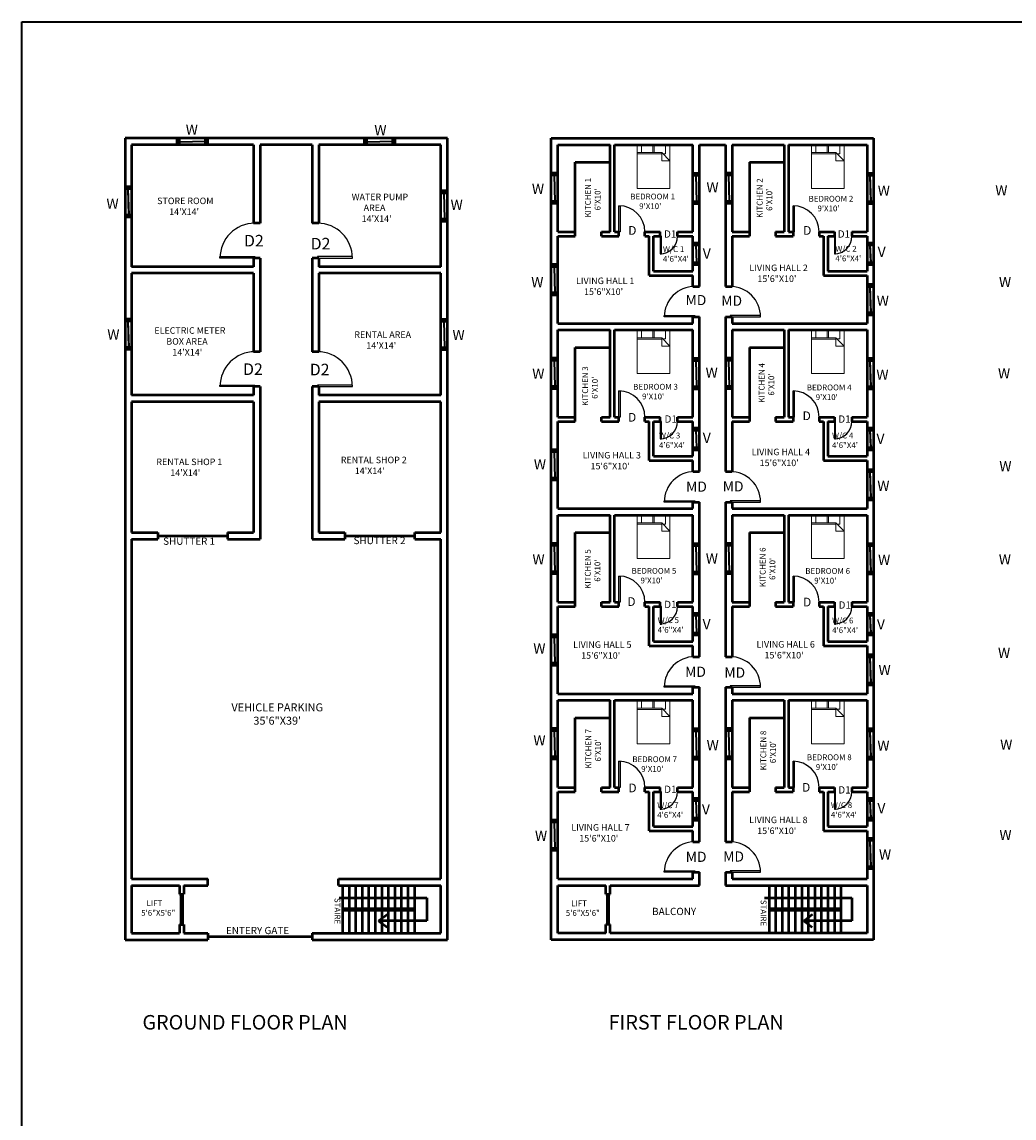
# Model space of a CAD drawing. Units: inches. Extents: x 9239 to 26065, y 6728 to 14611.
# Tile 10 of 12: x 23324 to 24691, y 13102 to 14611. Entities that reach past the tile are written whole.
import ezdxf

# ---------------------------------------------------------------- set-up
doc = ezdxf.new("R2010")
doc.units = ezdxf.units.IN
doc.header["$MEASUREMENT"] = 0
for name, color, linetype, lineweight in [('A-ANNO-TEXT', 7, 'Continuous', 18), ('A-ANNO-TTLB', 7, 'Continuous', 35), ('A-AREA-IDEN', 7, 'Continuous', 18), ('A-DOOR', 4, 'Continuous', 25), ('A-FURN', 8, 'Continuous', 18), ('A-GLAZ', 4, 'Continuous', 25), ('A-WALL', 7, 'Continuous', 50)]:
    doc.layers.add(name, color=color, linetype=linetype, lineweight=lineweight)
doc.styles.get("Standard").update_dxf_attribs({"font": 'arial.ttf'})

# ---------------------------------------------------------------- blocks, each defined once
blk = doc.blocks.new('*U10')
for p, q in [((0, 0), (0, -6)), ((36, 0), (36, -6))]:
    blk.add_line(p, q)
blk.add_lwpolyline([(0, 0), (0, 36), (1.75, 36), (1.75, 0)], close=True)
blk.add_arc((0, 0), 36, 0, 90)
blk = doc.blocks.new('*U34')
for p, q in [((0, 0), (0, 6)), ((24, 0), (24, 6))]:
    blk.add_line(p, q)
blk.add_lwpolyline([(0, 0), (0, -24), (1.75, -24), (1.75, 0)], close=True)
blk.add_arc((0, 0), 24, 270, 0)
blk = doc.blocks.new('*U33')
for p, q in [((-40, 0), (-40, 6)), ((0, 0), (0, 6))]:
    blk.add_line(p, q)
blk.add_lwpolyline([(0, 0), (0, -40), (-1.75, -40), (-1.75, 0)], close=True)
blk.add_arc((0, 0), 40, 180, 270)
blk = doc.blocks.new('*U35')
for p, q in [((0, 0), (0, -6)), ((-40, 0), (-40, -6))]:
    blk.add_line(p, q)
blk.add_lwpolyline([(0, 0), (0, 40), (-1.75, 40), (-1.75, 0)], close=True)
blk.add_arc((0, 0), 40, 90, 180)
blk = doc.blocks.new('*U36')
for p, q in [((-40, 0), (-40, 6)), ((0, 0), (0, 6))]:
    blk.add_line(p, q)
blk.add_lwpolyline([(0, 0), (0, -40), (-1.75, -40), (-1.75, 0)], close=True)
blk.add_arc((0, 0), 40, 180, 270)
blk = doc.blocks.new('Bed - Queen')
for p, q in [((0, -80.00003), (0, 0)), ((0, 0), (59.99999, 0)), ((59.99999, 0), (59.99999, -80.00003)), ((0, -14.4), (44.8, -14.4)), ((44.8, -16.8), (0, -16.8)), ((7.99999, -1.2), (28.79998, -1.2)), ((7.99999, -14.4), (7.99999, -1.2)), ((28.79998, -1.2), (28.79998, -14.4)), ((31.19999, -1.2), (51.99999, -1.2)), ((31.19999, -14.4), (31.19999, -1.2)), ((59.99999, -29.6), (44.8, -14.4)), ((44.8, -14.4), (44.8, -29.6)), ((51.99999, -16.4), (46.79936, -16.4)), ((51.99999, -1.2), (51.99999, -16.4)), ((44.8, -29.6), (59.99999, -29.6)), ((59.99999, -80.00003), (0, -80.00003))]:
    blk.add_line(p, q)
blk = doc.blocks.new('WIN-36')
for p, q in [((0, 1), (36, 1)), ((0, 0.5), (36, 0.5)), ((0, 0), (36, 0))]:
    blk.add_line(p, q)
blk = doc.blocks.new('WIN-24')
for p, q in [((0, 1), (24, 1)), ((0, 0.5), (24, 0.5)), ((0, 0), (24, 0))]:
    blk.add_line(p, q)

msp = doc.modelspace()

# ---------------------------------------------------------------- linework, layer by layer
at = {"layer": 'A-ANNO-TTLB'}
msp.add_lwpolyline([(23324.14, 14611.25), (26064.6, 14611.25), (26064.6, 11591.84), (23324.14, 11591.84)], close=True, dxfattribs=at)
at = {"layer": 'A-WALL'}
for p, q in [((23910.16, 14451.02), (23466.16, 14451.02)), ((23466.16, 14451.02), (23466.16, 13347.02)), ((23538.16, 14442.02), (23538.16, 14451.02)), ((23541.16, 14442.02), (23541.16, 14451.02)), ((23577.16, 14442.02), (23577.16, 14451.02)), ((23580.16, 14442.02), (23580.16, 14451.02)), ((23796.16, 14442.02), (23796.16, 14451.02)), ((23799.16, 14442.02), (23799.16, 14451.02)), ((23835.16, 14442.02), (23835.16, 14451.02)), ((23838.16, 14442.02), (23838.16, 14451.02)), ((23910.16, 13347.02), (23910.16, 14451.02)), ((24053.28, 14451.02), (24497.28, 14451.02)), ((24053.28, 13347.02), (24053.28, 14451.02)), ((24497.28, 14451.02), (24497.28, 13347.02)), ((23475.16, 14442.02), (23475.16, 14274.02)), ((23643.16, 14442.02), (23475.16, 14442.02)), ((23643.16, 14442.02), (23643.16, 14334.02)), ((23652.16, 14442.02), (23652.16, 14334.02)), ((23724.16, 14442.02), (23652.16, 14442.02)), ((23724.16, 14442.02), (23724.16, 14334.02)), ((23901.16, 14442.02), (23733.16, 14442.02)), ((23733.16, 14442.02), (23733.16, 14334.02)), ((23901.16, 14274.02), (23901.16, 14442.02)), ((24062.28, 14442.02), (24134.28, 14442.02)), ((24062.28, 14322.02), (24062.28, 14442.02)), ((24134.28, 14322.02), (24134.28, 14442.02)), ((24140.28, 14322.02), (24140.28, 14442.02)), ((24140.28, 14442.02), (24248.28, 14442.02)), ((24248.28, 14322.02), (24248.28, 14442.02)), ((24257.28, 14247.02), (24257.28, 14442.02)), ((24257.28, 14442.02), (24293.28, 14442.02)), ((24293.28, 14442.02), (24293.28, 14247.02)), ((24302.28, 14442.02), (24302.28, 14322.02)), ((24302.28, 14442.02), (24374.28, 14442.02)), ((24374.28, 14442.02), (24374.28, 14322.02)), ((24380.28, 14442.02), (24380.28, 14322.02)), ((24380.28, 14442.02), (24488.28, 14442.02)), ((24488.28, 14442.02), (24488.28, 14322.02)), ((24086.28, 14322.02), (24086.28, 14418.02)), ((24086.28, 14418.02), (24134.28, 14418.02)), ((24326.28, 14418.02), (24374.28, 14418.02)), ((24326.28, 14418.02), (24326.28, 14322.02)), ((24062.28, 14403.02), (24053.28, 14403.02)), ((24248.28, 14403.02), (24257.28, 14403.02)), ((24302.28, 14403.02), (24293.28, 14403.02)), ((24488.28, 14403.02), (24497.28, 14403.02)), ((24062.28, 14400.02), (24053.28, 14400.02)), ((24248.28, 14400.02), (24257.28, 14400.02)), ((24302.28, 14400.02), (24293.28, 14400.02)), ((24488.28, 14400.02), (24497.28, 14400.02)), ((23475.16, 14384.21), (23466.16, 14384.21)), ((23475.16, 14381.21), (23466.16, 14381.21)), ((23901.16, 14379.02), (23910.16, 14379.02)), ((23901.16, 14376.02), (23910.16, 14376.02)), ((24062.28, 14364.02), (24053.28, 14364.02)), ((24062.28, 14361.02), (24053.28, 14361.02)), ((24248.28, 14364.02), (24257.28, 14364.02)), ((24248.28, 14361.02), (24257.28, 14361.02)), ((24302.28, 14364.02), (24293.28, 14364.02)), ((24302.28, 14361.02), (24293.28, 14361.02)), ((24488.28, 14364.02), (24497.28, 14364.02)), ((24488.28, 14361.02), (24497.28, 14361.02)), ((23475.16, 14345.21), (23466.16, 14345.21)), ((23475.16, 14342.21), (23466.16, 14342.21)), ((23652.16, 14334.02), (23643.16, 14334.02)), ((23733.16, 14334.02), (23724.16, 14334.02)), ((23901.16, 14340.02), (23910.16, 14340.02)), ((23901.16, 14337.02), (23910.16, 14337.02)), ((24062.28, 14322.02), (24086.28, 14322.02)), ((24062.28, 14316.02), (24086.28, 14316.02)), ((24062.28, 14196.02), (24062.28, 14316.02)), ((24086.28, 14316.02), (24086.28, 14322.02)), ((24122.28, 14316.02), (24122.28, 14322.02)), ((24122.28, 14322.02), (24134.28, 14322.02)), ((24122.28, 14316.02), (24146.28, 14316.02)), ((24140.28, 14322.02), (24146.28, 14322.02)), ((24146.28, 14316.02), (24146.28, 14322.02)), ((24182.28, 14316.02), (24182.28, 14322.02)), ((24182.28, 14322.02), (24203.28, 14322.02)), ((24182.28, 14316.02), (24188.28, 14316.02)), ((24188.28, 14262.02), (24188.28, 14316.02)), ((24194.28, 14268.02), (24194.28, 14316.02)), ((24194.28, 14316.02), (24203.28, 14316.02)), ((24203.28, 14316.02), (24203.28, 14322.02)), ((24227.28, 14316.02), (24227.28, 14322.02)), ((24227.28, 14322.02), (24248.28, 14322.02)), ((24227.28, 14316.02), (24248.28, 14316.02)), ((24248.28, 14268.02), (24248.28, 14316.02)), ((24302.28, 14322.02), (24326.28, 14322.02)), ((24302.28, 14316.02), (24326.28, 14316.02)), ((24302.28, 14316.02), (24302.28, 14247.02)), ((24326.28, 14322.02), (24326.28, 14316.02)), ((24362.28, 14322.02), (24362.28, 14316.02)), ((24362.28, 14322.02), (24374.28, 14322.02)), ((24362.28, 14316.02), (24386.28, 14316.02)), ((24380.28, 14322.02), (24386.28, 14322.02)), ((24386.28, 14322.02), (24386.28, 14316.02)), ((24422.28, 14322.02), (24422.28, 14316.02)), ((24422.28, 14322.02), (24443.28, 14322.02)), ((24422.28, 14316.02), (24428.28, 14316.02)), ((24428.28, 14316.02), (24428.28, 14262.02)), ((24434.28, 14316.02), (24434.28, 14268.02)), ((24434.28, 14316.02), (24443.28, 14316.02)), ((24443.28, 14322.02), (24443.28, 14316.02)), ((24467.28, 14322.02), (24467.28, 14316.02)), ((24467.28, 14322.02), (24488.28, 14322.02)), ((24467.28, 14316.02), (24488.28, 14316.02)), ((24488.28, 14316.02), (24488.28, 14268.02)), ((24248.28, 14307.02), (24257.28, 14307.02)), ((24248.28, 14304.02), (24257.28, 14304.02)), ((24488.28, 14307.02), (24497.28, 14307.02)), ((24488.28, 14304.02), (24497.28, 14304.02)), ((23652.16, 14286.02), (23643.16, 14286.02)), ((23643.16, 14286.02), (23643.16, 14274.02)), ((23652.16, 14286.02), (23652.16, 14157.02)), ((23733.16, 14286.02), (23724.16, 14286.02)), ((23724.16, 14286.02), (23724.16, 14157.02)), ((23733.16, 14286.02), (23733.16, 14274.02)), ((23643.16, 14274.02), (23475.16, 14274.02)), ((23901.16, 14274.02), (23733.16, 14274.02)), ((24062.28, 14277.02), (24053.28, 14277.02)), ((24062.28, 14274.02), (24053.28, 14274.02)), ((24194.28, 14268.02), (24248.28, 14268.02)), ((24248.28, 14280.02), (24257.28, 14280.02)), ((24248.28, 14277.02), (24257.28, 14277.02)), ((24434.28, 14268.02), (24488.28, 14268.02)), ((24488.28, 14280.02), (24497.28, 14280.02)), ((24488.28, 14277.02), (24497.28, 14277.02)), ((23643.16, 14265.02), (23475.16, 14265.02)), ((23475.16, 14265.02), (23475.16, 14097.02)), ((23643.16, 14265.02), (23643.16, 14157.02)), ((23901.16, 14265.02), (23733.16, 14265.02)), ((23733.16, 14265.02), (23733.16, 14157.02)), ((23901.16, 14097.02), (23901.16, 14265.02)), ((24188.28, 14262.02), (24248.28, 14262.02)), ((24248.28, 14247.02), (24248.28, 14262.02)), ((24428.28, 14262.02), (24488.28, 14262.02)), ((24488.28, 14262.02), (24488.28, 14196.02)), ((24062.28, 14238.02), (24053.28, 14238.02)), ((24248.28, 14247.02), (24257.28, 14247.02)), ((24293.28, 14247.02), (24302.28, 14247.02)), ((24488.28, 14250.02), (24497.28, 14250.02)), ((24488.28, 14247.02), (24497.28, 14247.02)), ((24062.28, 14235.02), (24053.28, 14235.02)), ((24488.28, 14211.02), (24497.28, 14211.02)), ((24488.28, 14208.02), (24497.28, 14208.02)), ((23475.16, 14202.02), (23466.16, 14202.02)), ((23475.16, 14199.02), (23466.16, 14199.02)), ((23901.16, 14202.02), (23910.16, 14202.02)), ((23901.16, 14199.02), (23910.16, 14199.02)), ((24062.28, 14196.02), (24248.28, 14196.02)), ((24248.28, 14205.02), (24257.28, 14205.02)), ((24248.28, 14196.02), (24248.28, 14205.02)), ((24257.28, 13992.02), (24257.28, 14205.02)), ((24293.28, 14205.02), (24302.28, 14205.02)), ((24293.28, 14205.02), (24293.28, 13992.02)), ((24302.28, 14205.02), (24302.28, 14196.02)), ((24302.28, 14196.02), (24488.28, 14196.02)), ((24062.28, 14187.02), (24134.28, 14187.02)), ((24062.28, 14067.02), (24062.28, 14187.02)), ((24134.28, 14067.02), (24134.28, 14187.02)), ((24140.28, 14067.02), (24140.28, 14187.02)), ((24140.28, 14187.02), (24248.28, 14187.02)), ((24248.28, 14067.02), (24248.28, 14187.02)), ((24302.28, 14187.02), (24374.28, 14187.02)), ((24302.28, 14187.02), (24302.28, 14067.02)), ((24374.28, 14187.02), (24374.28, 14067.02)), ((24380.28, 14187.02), (24380.28, 14067.02)), ((24380.28, 14187.02), (24488.28, 14187.02)), ((24488.28, 14187.02), (24488.28, 14067.02)), ((23475.16, 14163.02), (23466.16, 14163.02)), ((23901.16, 14163.02), (23910.16, 14163.02)), ((24086.28, 14067.02), (24086.28, 14163.02)), ((24086.28, 14163.02), (24134.28, 14163.02)), ((24326.28, 14163.02), (24326.28, 14067.02)), ((24326.28, 14163.02), (24374.28, 14163.02)), ((23475.16, 14160.02), (23466.16, 14160.02)), ((23652.16, 14157.02), (23643.16, 14157.02)), ((23733.16, 14157.02), (23724.16, 14157.02)), ((23901.16, 14160.02), (23910.16, 14160.02)), ((24062.28, 14148.02), (24053.28, 14148.02)), ((24248.28, 14148.02), (24257.28, 14148.02)), ((24302.28, 14148.02), (24293.28, 14148.02)), ((24488.28, 14148.02), (24497.28, 14148.02)), ((24062.28, 14145.02), (24053.28, 14145.02)), ((24248.28, 14145.02), (24257.28, 14145.02)), ((24302.28, 14145.02), (24293.28, 14145.02)), ((24488.28, 14145.02), (24497.28, 14145.02)), ((23652.16, 14109.02), (23643.16, 14109.02)), ((23643.16, 14109.02), (23643.16, 14097.02)), ((23652.16, 14109.02), (23652.16, 13899.02)), ((23733.16, 14109.02), (23724.16, 14109.02)), ((23724.16, 14109.02), (23724.16, 13899.02)), ((23733.16, 14109.02), (23733.16, 14097.02)), ((24062.28, 14109.02), (24053.28, 14109.02)), ((24062.28, 14106.02), (24053.28, 14106.02)), ((24248.28, 14109.02), (24257.28, 14109.02)), ((24248.28, 14106.02), (24257.28, 14106.02)), ((24302.28, 14109.02), (24293.28, 14109.02)), ((24302.28, 14106.02), (24293.28, 14106.02)), ((24488.28, 14109.02), (24497.28, 14109.02)), ((24488.28, 14106.02), (24497.28, 14106.02)), ((23643.16, 14097.02), (23475.16, 14097.02)), ((23643.16, 14088.02), (23475.16, 14088.02)), ((23475.16, 14088.02), (23475.16, 13908.02)), ((23643.16, 14088.02), (23643.16, 13908.02)), ((23901.16, 14097.02), (23733.16, 14097.02)), ((23901.16, 14088.02), (23733.16, 14088.02)), ((23733.16, 14088.02), (23733.16, 13908.02)), ((23901.16, 13908.02), (23901.16, 14088.02)), ((24062.28, 14067.02), (24086.28, 14067.02)), ((24062.28, 14061.02), (24086.28, 14061.02)), ((24062.28, 13941.02), (24062.28, 14061.02)), ((24086.28, 14061.02), (24086.28, 14067.02)), ((24122.28, 14061.02), (24122.28, 14067.02)), ((24122.28, 14067.02), (24134.28, 14067.02)), ((24122.28, 14061.02), (24146.28, 14061.02)), ((24140.28, 14067.02), (24146.28, 14067.02)), ((24146.28, 14061.02), (24146.28, 14067.02)), ((24182.28, 14061.02), (24182.28, 14067.02)), ((24182.28, 14067.02), (24203.28, 14067.02)), ((24182.28, 14061.02), (24188.28, 14061.02)), ((24188.28, 14007.02), (24188.28, 14061.02)), ((24194.28, 14013.02), (24194.28, 14061.02)), ((24194.28, 14061.02), (24203.28, 14061.02)), ((24203.28, 14061.02), (24203.28, 14067.02)), ((24227.28, 14061.02), (24227.28, 14067.02)), ((24227.28, 14067.02), (24248.28, 14067.02)), ((24227.28, 14061.02), (24248.28, 14061.02)), ((24248.28, 14013.02), (24248.28, 14061.02)), ((24302.28, 14067.02), (24326.28, 14067.02)), ((24302.28, 14061.02), (24326.28, 14061.02)), ((24302.28, 14061.02), (24302.28, 13992.02)), ((24326.28, 14067.02), (24326.28, 14061.02)), ((24362.28, 14067.02), (24362.28, 14061.02)), ((24362.28, 14067.02), (24374.28, 14067.02)), ((24362.28, 14061.02), (24386.28, 14061.02)), ((24380.28, 14067.02), (24386.28, 14067.02)), ((24386.28, 14067.02), (24386.28, 14061.02)), ((24422.28, 14067.02), (24422.28, 14061.02)), ((24422.28, 14067.02), (24443.28, 14067.02)), ((24422.28, 14061.02), (24428.28, 14061.02)), ((24428.28, 14061.02), (24428.28, 14007.02)), ((24434.28, 14061.02), (24434.28, 14013.02)), ((24434.28, 14061.02), (24443.28, 14061.02)), ((24443.28, 14067.02), (24443.28, 14061.02)), ((24467.28, 14067.02), (24467.28, 14061.02)), ((24467.28, 14067.02), (24488.28, 14067.02)), ((24467.28, 14061.02), (24488.28, 14061.02)), ((24488.28, 14061.02), (24488.28, 14013.02)), ((24248.28, 14052.02), (24257.28, 14052.02)), ((24248.28, 14049.02), (24257.28, 14049.02)), ((24488.28, 14052.02), (24497.28, 14052.02)), ((24488.28, 14049.02), (24497.28, 14049.02)), ((24062.28, 14022.02), (24053.28, 14022.02)), ((24062.28, 14019.02), (24053.28, 14019.02)), ((24194.28, 14013.02), (24248.28, 14013.02)), ((24248.28, 14025.02), (24257.28, 14025.02)), ((24248.28, 14022.02), (24257.28, 14022.02)), ((24434.28, 14013.02), (24488.28, 14013.02)), ((24488.28, 14025.02), (24497.28, 14025.02)), ((24488.28, 14022.02), (24497.28, 14022.02)), ((24188.28, 14007.02), (24248.28, 14007.02)), ((24248.28, 13992.02), (24248.28, 14007.02)), ((24428.28, 14007.02), (24488.28, 14007.02)), ((24488.28, 14007.02), (24488.28, 13941.02)), ((24488.28, 13995.02), (24497.28, 13995.02)), ((24062.28, 13983.02), (24053.28, 13983.02)), ((24062.28, 13980.02), (24053.28, 13980.02)), ((24248.28, 13992.02), (24257.28, 13992.02)), ((24293.28, 13992.02), (24302.28, 13992.02)), ((24488.28, 13992.02), (24497.28, 13992.02)), ((24248.28, 13950.02), (24257.28, 13950.02)), ((24248.28, 13941.02), (24248.28, 13950.02)), ((24257.28, 13737.02), (24257.28, 13950.02)), ((24293.28, 13950.02), (24302.28, 13950.02)), ((24293.28, 13950.02), (24293.28, 13737.02)), ((24302.28, 13950.02), (24302.28, 13941.02)), ((24488.28, 13956.02), (24497.28, 13956.02)), ((24488.28, 13953.02), (24497.28, 13953.02)), ((24062.28, 13941.02), (24248.28, 13941.02)), ((24302.28, 13941.02), (24488.28, 13941.02)), ((24062.28, 13932.02), (24134.28, 13932.02)), ((24062.28, 13812.02), (24062.28, 13932.02)), ((24134.28, 13812.02), (24134.28, 13932.02)), ((24140.28, 13812.02), (24140.28, 13932.02)), ((24140.28, 13932.02), (24248.28, 13932.02)), ((24248.28, 13812.02), (24248.28, 13932.02)), ((24302.28, 13932.02), (24374.28, 13932.02)), ((24302.28, 13932.02), (24302.28, 13812.02)), ((24374.28, 13932.02), (24374.28, 13812.02)), ((24380.28, 13932.02), (24380.28, 13812.02)), ((24380.28, 13932.02), (24488.28, 13932.02)), ((24488.28, 13932.02), (24488.28, 13812.02)), ((23475.16, 13908.02), (23511.16, 13908.02)), ((23511.16, 13908.02), (23511.16, 13899.02)), ((23607.16, 13908.02), (23607.16, 13899.02)), ((23607.16, 13908.02), (23643.16, 13908.02)), ((23733.16, 13908.02), (23769.16, 13908.02)), ((23769.16, 13908.02), (23769.16, 13899.02)), ((23865.16, 13899.02), (23865.16, 13908.02)), ((23865.16, 13908.02), (23901.16, 13908.02)), ((24086.28, 13812.02), (24086.28, 13908.02)), ((24086.28, 13908.02), (24134.28, 13908.02)), ((24326.28, 13908.02), (24326.28, 13812.02)), ((24326.28, 13908.02), (24374.28, 13908.02)), ((23475.16, 13899.02), (23511.16, 13899.02)), ((23475.16, 13899.02), (23475.16, 13431.02)), ((23511.16, 13903.52), (23607.16, 13903.52)), ((23607.16, 13899.02), (23652.16, 13899.02)), ((23724.16, 13899.02), (23769.16, 13899.02)), ((23769.16, 13903.52), (23865.16, 13903.52)), ((23865.16, 13899.02), (23901.16, 13899.02)), ((23901.16, 13431.02), (23901.16, 13899.02)), ((24062.28, 13893.02), (24053.28, 13893.02)), ((24062.28, 13890.02), (24053.28, 13890.02)), ((24248.28, 13893.02), (24257.28, 13893.02)), ((24248.28, 13890.02), (24257.28, 13890.02)), ((24302.28, 13893.02), (24293.28, 13893.02)), ((24302.28, 13890.02), (24293.28, 13890.02)), ((24488.28, 13893.02), (24497.28, 13893.02)), ((24488.28, 13890.02), (24497.28, 13890.02)), ((24062.28, 13854.02), (24053.28, 13854.02)), ((24062.28, 13851.02), (24053.28, 13851.02)), ((24248.28, 13854.02), (24257.28, 13854.02)), ((24248.28, 13851.02), (24257.28, 13851.02)), ((24302.28, 13854.02), (24293.28, 13854.02)), ((24302.28, 13851.02), (24293.28, 13851.02)), ((24488.28, 13854.02), (24497.28, 13854.02)), ((24488.28, 13851.02), (24497.28, 13851.02)), ((24062.28, 13812.02), (24086.28, 13812.02)), ((24062.28, 13806.02), (24086.28, 13806.02)), ((24062.28, 13686.02), (24062.28, 13806.02)), ((24086.28, 13806.02), (24086.28, 13812.02)), ((24122.28, 13806.02), (24122.28, 13812.02)), ((24122.28, 13812.02), (24134.28, 13812.02)), ((24122.28, 13806.02), (24146.28, 13806.02)), ((24140.28, 13812.02), (24146.28, 13812.02)), ((24146.28, 13806.02), (24146.28, 13812.02)), ((24182.28, 13806.02), (24182.28, 13812.02)), ((24182.28, 13812.02), (24203.28, 13812.02)), ((24182.28, 13806.02), (24188.28, 13806.02)), ((24188.28, 13752.02), (24188.28, 13806.02)), ((24194.28, 13758.02), (24194.28, 13806.02)), ((24194.28, 13806.02), (24203.28, 13806.02)), ((24203.28, 13806.02), (24203.28, 13812.02)), ((24227.28, 13806.02), (24227.28, 13812.02)), ((24227.28, 13812.02), (24248.28, 13812.02)), ((24227.28, 13806.02), (24248.28, 13806.02)), ((24248.28, 13758.02), (24248.28, 13806.02)), ((24302.28, 13812.02), (24326.28, 13812.02)), ((24302.28, 13806.02), (24326.28, 13806.02)), ((24302.28, 13806.02), (24302.28, 13737.02)), ((24326.28, 13812.02), (24326.28, 13806.02)), ((24362.28, 13812.02), (24362.28, 13806.02)), ((24362.28, 13812.02), (24374.28, 13812.02)), ((24362.28, 13806.02), (24386.28, 13806.02)), ((24380.28, 13812.02), (24386.28, 13812.02)), ((24386.28, 13812.02), (24386.28, 13806.02)), ((24422.28, 13812.02), (24422.28, 13806.02)), ((24422.28, 13812.02), (24443.28, 13812.02)), ((24422.28, 13806.02), (24428.28, 13806.02)), ((24428.28, 13806.02), (24428.28, 13752.02)), ((24434.28, 13806.02), (24434.28, 13758.02)), ((24434.28, 13806.02), (24443.28, 13806.02)), ((24443.28, 13812.02), (24443.28, 13806.02)), ((24467.28, 13812.02), (24467.28, 13806.02)), ((24467.28, 13812.02), (24488.28, 13812.02)), ((24467.28, 13806.02), (24488.28, 13806.02)), ((24488.28, 13806.02), (24488.28, 13758.02)), ((24248.28, 13797.02), (24257.28, 13797.02)), ((24248.28, 13794.02), (24257.28, 13794.02)), ((24488.28, 13797.02), (24497.28, 13797.02)), ((24488.28, 13794.02), (24497.28, 13794.02)), ((24248.28, 13770.02), (24257.28, 13770.02)), ((24488.28, 13770.02), (24497.28, 13770.02)), ((24062.28, 13767.02), (24053.28, 13767.02)), ((24062.28, 13764.02), (24053.28, 13764.02)), ((24194.28, 13758.02), (24248.28, 13758.02)), ((24248.28, 13767.02), (24257.28, 13767.02)), ((24434.28, 13758.02), (24488.28, 13758.02)), ((24488.28, 13767.02), (24497.28, 13767.02)), ((24188.28, 13752.02), (24248.28, 13752.02)), ((24248.28, 13737.02), (24248.28, 13752.02)), ((24428.28, 13752.02), (24488.28, 13752.02)), ((24488.28, 13752.02), (24488.28, 13686.02)), ((24488.28, 13740.02), (24497.28, 13740.02)), ((24062.28, 13728.02), (24053.28, 13728.02)), ((24062.28, 13725.02), (24053.28, 13725.02)), ((24248.28, 13737.02), (24257.28, 13737.02)), ((24293.28, 13737.02), (24302.28, 13737.02)), ((24488.28, 13737.02), (24497.28, 13737.02)), ((24248.28, 13695.02), (24257.28, 13695.02)), ((24248.28, 13686.02), (24248.28, 13695.02)), ((24257.28, 13482.02), (24257.28, 13695.02)), ((24293.28, 13695.02), (24302.28, 13695.02)), ((24293.28, 13695.02), (24293.28, 13482.02)), ((24302.28, 13695.02), (24302.28, 13686.02)), ((24488.28, 13701.02), (24497.28, 13701.02)), ((24488.28, 13698.02), (24497.28, 13698.02)), ((24062.28, 13686.02), (24248.28, 13686.02)), ((24302.28, 13686.02), (24488.28, 13686.02)), ((24062.28, 13677.02), (24134.28, 13677.02)), ((24062.28, 13557.02), (24062.28, 13677.02)), ((24134.28, 13557.02), (24134.28, 13677.02)), ((24140.28, 13557.02), (24140.28, 13677.02)), ((24140.28, 13677.02), (24248.28, 13677.02)), ((24248.28, 13557.02), (24248.28, 13677.02)), ((24302.28, 13677.02), (24374.28, 13677.02)), ((24302.28, 13677.02), (24302.28, 13557.02)), ((24374.28, 13677.02), (24374.28, 13557.02)), ((24380.28, 13677.02), (24380.28, 13557.02)), ((24380.28, 13677.02), (24488.28, 13677.02)), ((24488.28, 13677.02), (24488.28, 13557.02)), ((24086.28, 13557.02), (24086.28, 13653.02)), ((24086.28, 13653.02), (24134.28, 13653.02)), ((24326.28, 13653.02), (24326.28, 13557.02)), ((24326.28, 13653.02), (24374.28, 13653.02)), ((24062.28, 13638.02), (24053.28, 13638.02)), ((24062.28, 13635.02), (24053.28, 13635.02)), ((24248.28, 13638.02), (24257.28, 13638.02)), ((24248.28, 13635.02), (24257.28, 13635.02)), ((24302.28, 13638.02), (24293.28, 13638.02)), ((24302.28, 13635.02), (24293.28, 13635.02)), ((24488.28, 13638.02), (24497.28, 13638.02)), ((24488.28, 13635.02), (24497.28, 13635.02)), ((24062.28, 13599.02), (24053.28, 13599.02)), ((24062.28, 13596.02), (24053.28, 13596.02)), ((24248.28, 13599.02), (24257.28, 13599.02)), ((24248.28, 13596.02), (24257.28, 13596.02)), ((24302.28, 13599.02), (24293.28, 13599.02)), ((24302.28, 13596.02), (24293.28, 13596.02)), ((24488.28, 13599.02), (24497.28, 13599.02)), ((24488.28, 13596.02), (24497.28, 13596.02)), ((24062.28, 13557.02), (24086.28, 13557.02)), ((24062.28, 13551.02), (24086.28, 13551.02)), ((24062.28, 13431.02), (24062.28, 13551.02)), ((24086.28, 13551.02), (24086.28, 13557.02)), ((24122.28, 13551.02), (24122.28, 13557.02)), ((24122.28, 13557.02), (24134.28, 13557.02)), ((24122.28, 13551.02), (24146.28, 13551.02)), ((24140.28, 13557.02), (24146.28, 13557.02)), ((24146.28, 13551.02), (24146.28, 13557.02)), ((24182.28, 13551.02), (24182.28, 13557.02)), ((24182.28, 13557.02), (24203.28, 13557.02)), ((24182.28, 13551.02), (24188.28, 13551.02)), ((24188.28, 13497.02), (24188.28, 13551.02)), ((24194.28, 13503.02), (24194.28, 13551.02)), ((24194.28, 13551.02), (24203.28, 13551.02)), ((24203.28, 13551.02), (24203.28, 13557.02)), ((24227.28, 13551.02), (24227.28, 13557.02)), ((24227.28, 13557.02), (24248.28, 13557.02)), ((24227.28, 13551.02), (24248.28, 13551.02)), ((24248.28, 13503.02), (24248.28, 13551.02)), ((24302.28, 13557.02), (24326.28, 13557.02)), ((24302.28, 13551.02), (24326.28, 13551.02)), ((24302.28, 13551.02), (24302.28, 13482.02)), ((24326.28, 13557.02), (24326.28, 13551.02)), ((24362.28, 13557.02), (24362.28, 13551.02)), ((24362.28, 13557.02), (24374.28, 13557.02)), ((24362.28, 13551.02), (24386.28, 13551.02)), ((24380.28, 13557.02), (24386.28, 13557.02)), ((24386.28, 13557.02), (24386.28, 13551.02)), ((24422.28, 13557.02), (24422.28, 13551.02)), ((24422.28, 13557.02), (24443.28, 13557.02)), ((24422.28, 13551.02), (24428.28, 13551.02)), ((24428.28, 13551.02), (24428.28, 13497.02)), ((24434.28, 13551.02), (24434.28, 13503.02)), ((24434.28, 13551.02), (24443.28, 13551.02)), ((24443.28, 13557.02), (24443.28, 13551.02)), ((24467.28, 13557.02), (24467.28, 13551.02)), ((24467.28, 13557.02), (24488.28, 13557.02)), ((24467.28, 13551.02), (24488.28, 13551.02)), ((24488.28, 13551.02), (24488.28, 13503.02)), ((24248.28, 13542.02), (24257.28, 13542.02)), ((24248.28, 13539.02), (24257.28, 13539.02)), ((24488.28, 13542.02), (24497.28, 13542.02)), ((24488.28, 13539.02), (24497.28, 13539.02)), ((24062.28, 13512.02), (24053.28, 13512.02)), ((24248.28, 13515.02), (24257.28, 13515.02)), ((24248.28, 13512.02), (24257.28, 13512.02)), ((24488.28, 13515.02), (24497.28, 13515.02)), ((24488.28, 13512.02), (24497.28, 13512.02)), ((24062.28, 13509.02), (24053.28, 13509.02)), ((24188.28, 13497.02), (24248.28, 13497.02)), ((24194.28, 13503.02), (24248.28, 13503.02)), ((24248.28, 13482.02), (24248.28, 13497.02)), ((24428.28, 13497.02), (24488.28, 13497.02)), ((24434.28, 13503.02), (24488.28, 13503.02)), ((24488.28, 13497.02), (24488.28, 13431.02)), ((24248.28, 13482.02), (24257.28, 13482.02)), ((24293.28, 13482.02), (24302.28, 13482.02)), ((24488.28, 13487.16), (24497.28, 13487.16)), ((24488.28, 13484.16), (24497.28, 13484.16)), ((24062.28, 13473.02), (24053.28, 13473.02)), ((24062.28, 13470.02), (24053.28, 13470.02)), ((24248.28, 13431.02), (24248.28, 13440.02)), ((24248.28, 13440.02), (24257.28, 13440.02)), ((24257.28, 13422.02), (24257.28, 13440.02)), ((24293.28, 13440.02), (24302.28, 13440.02)), ((24293.28, 13440.02), (24293.28, 13422.02)), ((24302.28, 13440.02), (24302.28, 13431.02)), ((24488.28, 13448.16), (24497.28, 13448.16)), ((24488.28, 13445.16), (24497.28, 13445.16)), ((23475.16, 13431.02), (23580.16, 13431.02)), ((23475.16, 13422.02), (23541.16, 13422.02)), ((23475.16, 13422.02), (23475.16, 13356.02)), ((23541.16, 13422.02), (23541.16, 13410.02)), ((23547.16, 13422.02), (23547.16, 13410.02)), ((23547.16, 13422.02), (23580.16, 13422.02)), ((23580.16, 13422.02), (23580.16, 13431.02)), ((23760.16, 13431.02), (23901.16, 13431.02)), ((23760.16, 13422.02), (23760.16, 13431.02)), ((23760.16, 13422.02), (23901.16, 13422.02)), ((23766.16, 13356.02), (23766.16, 13422.02)), ((23775.16, 13390.02), (23775.16, 13422.02)), ((23784.16, 13390.02), (23784.16, 13422.02)), ((23793.16, 13390.02), (23793.16, 13422.02)), ((23802.16, 13390.02), (23802.16, 13422.02)), ((23811.16, 13390.02), (23811.16, 13422.02)), ((23820.16, 13390.02), (23820.16, 13422.02)), ((23829.16, 13390.02), (23829.16, 13422.02)), ((23838.16, 13390.02), (23838.16, 13422.02)), ((23847.16, 13390.02), (23847.16, 13422.02)), ((23856.16, 13390.02), (23856.16, 13422.02)), ((23865.16, 13356.02), (23865.16, 13422.02)), ((23901.16, 13356.02), (23901.16, 13422.02)), ((24062.28, 13431.02), (24248.28, 13431.02)), ((24062.28, 13356.02), (24062.28, 13422.02)), ((24062.28, 13422.02), (24128.28, 13422.02)), ((24128.28, 13410.02), (24128.28, 13422.02)), ((24134.28, 13422.02), (24257.28, 13422.02)), ((24134.28, 13410.02), (24134.28, 13422.02)), ((24293.28, 13422.02), (24488.28, 13422.02)), ((24302.28, 13431.02), (24488.28, 13431.02)), ((24353.28, 13422.02), (24353.28, 13356.02)), ((24362.28, 13422.02), (24362.28, 13390.02)), ((24371.28, 13422.02), (24371.28, 13390.02)), ((24380.28, 13422.02), (24380.28, 13390.02)), ((24389.28, 13422.02), (24389.28, 13390.02)), ((24398.28, 13422.02), (24398.28, 13390.02)), ((24407.28, 13422.02), (24407.28, 13390.02)), ((24416.28, 13422.02), (24416.28, 13390.02)), ((24425.28, 13422.02), (24425.28, 13390.02)), ((24434.28, 13422.02), (24434.28, 13390.02)), ((24443.28, 13422.02), (24443.28, 13390.02)), ((24452.28, 13422.02), (24452.28, 13356.02)), ((24488.28, 13422.02), (24488.28, 13356.02)), ((23541.16, 13410.02), (23547.16, 13410.02)), ((23543.16, 13410.02), (23543.16, 13368.02)), ((23545.16, 13410.02), (23545.16, 13368.02)), ((24128.28, 13410.02), (24134.28, 13410.02)), ((24130.28, 13410.02), (24130.28, 13368.02)), ((24132.28, 13410.02), (24132.28, 13368.02)), ((23761.25, 13404.84), (23881.69, 13404.84)), ((23881.69, 13404.84), (23881.69, 13373.34)), ((24346.8, 13404.84), (24467.24, 13404.84)), ((24467.24, 13404.84), (24467.24, 13373.34)), ((23766.16, 13390.02), (23865.16, 13390.02)), ((23766.16, 13388.02), (23865.16, 13388.02)), ((23775.16, 13356.02), (23775.16, 13388.02)), ((23784.16, 13356.02), (23784.16, 13388.02)), ((23793.16, 13356.02), (23793.16, 13388.02)), ((23802.16, 13356.02), (23802.16, 13388.02)), ((23811.16, 13356.02), (23811.16, 13388.02)), ((23815.48, 13373.34), (23827.54, 13382.6)), ((23820.16, 13356.02), (23820.16, 13388.02)), ((23829.16, 13356.02), (23829.16, 13388.02)), ((23838.16, 13356.02), (23838.16, 13388.02)), ((23847.16, 13356.02), (23847.16, 13388.02)), ((23856.16, 13356.02), (23856.16, 13388.02)), ((24353.28, 13390.02), (24452.28, 13390.02)), ((24353.28, 13388.02), (24452.28, 13388.02)), ((24362.28, 13388.02), (24362.28, 13356.02)), ((24371.28, 13388.02), (24371.28, 13356.02)), ((24380.28, 13388.02), (24380.28, 13356.02)), ((24389.28, 13388.02), (24389.28, 13356.02)), ((24398.28, 13388.02), (24398.28, 13356.02)), ((24401.03, 13373.34), (24413.09, 13382.6)), ((24407.28, 13388.02), (24407.28, 13356.02)), ((24416.28, 13388.02), (24416.28, 13356.02)), ((24425.28, 13388.02), (24425.28, 13356.02)), ((24434.28, 13388.02), (24434.28, 13356.02)), ((24443.28, 13388.02), (24443.28, 13356.02)), ((23541.16, 13368.02), (23547.16, 13368.02)), ((23541.16, 13368.02), (23541.16, 13356.02)), ((23547.16, 13368.02), (23547.16, 13356.02)), ((23881.69, 13373.34), (23815.48, 13373.34)), ((23815.48, 13373.34), (23827.26, 13364.58)), ((24128.28, 13356.02), (24128.28, 13368.02)), ((24134.28, 13368.02), (24128.28, 13368.02)), ((24134.28, 13356.02), (24134.28, 13368.02)), ((24467.24, 13373.34), (24401.03, 13373.34)), ((24401.03, 13373.34), (24412.81, 13364.58)), ((23466.16, 13347.02), (23580.16, 13347.02)), ((23475.16, 13356.02), (23541.16, 13356.02)), ((23547.16, 13356.02), (23580.16, 13356.02)), ((23580.16, 13356.02), (23580.16, 13347.02)), ((23580.16, 13351.52), (23724.16, 13351.52)), ((23724.16, 13356.02), (23901.16, 13356.02)), ((23724.16, 13356.02), (23724.16, 13347.02)), ((23724.16, 13347.02), (23910.16, 13347.02)), ((24497.28, 13347.02), (24053.28, 13347.02)), ((24128.28, 13356.02), (24062.28, 13356.02)), ((24488.28, 13356.02), (24134.28, 13356.02))]:
    msp.add_line(p, q, dxfattribs=at)

# ---------------------------------------------------------------- block references
at = {"layer": 'A-DOOR'}
for name, p in [('*U10', (24146.28, 14322.02)), ('*U10', (24386.28, 14322.02)), ('*U34', (24203.28, 14316.02)), ('*U34', (24443.28, 14316.02)), ('*U10', (24146.28, 14067.02)), ('*U10', (24386.28, 14067.02)), ('*U34', (24203.28, 14061.02)), ('*U34', (24443.28, 14061.02)), ('*U10', (24146.28, 13812.02)), ('*U10', (24386.28, 13812.02)), ('*U34', (24203.28, 13806.02)), ('*U34', (24443.28, 13806.02)), ('*U10', (24146.28, 13557.02)), ('*U10', (24386.28, 13557.02)), ('*U34', (24203.28, 13551.02)), ('*U34', (24443.28, 13551.02))]:
    msp.add_blockref(name, p, dxfattribs=at)
at = {"layer": 'A-DOOR', "rotation": 270}
for name, p, xscale, yscale, zscale in [('*U36', (23644.96, 14286.02), 1.199999999999999, 1.199999999999999, 1.199999999999999), ('*U35', (23731.36, 14286.02), 1.199999999999999, 1.199999999999999, 1.199999999999999), ('*U33', (24250.98, 14205.02), 1.05, 1.05, 1.05), ('*U35', (24299.58, 14205.02), 1.05, 1.05, 1.05), ('*U36', (23644.96, 14109.02), 1.199999999999999, 1.199999999999999, 1.199999999999999), ('*U35', (23731.36, 14109.02), 1.199999999999999, 1.199999999999999, 1.199999999999999), ('*U33', (24250.98, 13950.02), 1.05, 1.05, 1.05), ('*U35', (24299.58, 13950.02), 1.05, 1.05, 1.05), ('*U33', (24250.98, 13695.02), 1.049999999999997, 1.049999999999997, 1.049999999999997), ('*U35', (24299.58, 13695.02), 1.05, 1.05, 1.05), ('*U33', (24250.98, 13440.02), 1.049999999999954, 1.049999999999954, 1.049999999999954), ('*U35', (24299.58, 13440.02), 1.05, 1.05, 1.05)]:
    msp.add_blockref(name, p, dxfattribs=dict(at, xscale=xscale, yscale=yscale, zscale=zscale))
at = {"layer": 'A-FURN', "xscale": 0.75, "yscale": 0.75, "zscale": 0.75}
for p in [(24171.78, 14442.02), (24411.78, 14442.02), (24171.78, 14187.02), (24411.78, 14187.02), (24171.78, 13932.02), (24411.78, 13932.02), (24171.78, 13677.02), (24411.78, 13677.02)]:
    msp.add_blockref('Bed - Queen', p, dxfattribs=at)
at = {"layer": 'A-GLAZ'}
for name, p, rotation in [('WIN-36', (23541.18, 14445.52), 1.591140271200308), ('WIN-36', (23799.18, 14445.52), 1.591140271200308), ('WIN-36', (24056.78, 14400), 271.5911402711772), ('WIN-36', (24251.78, 14400), 271.5911402712003), ('WIN-36', (24296.78, 14400), 271.5911402712003), ('WIN-36', (24491.78, 14400), 271.5911402712003), ('WIN-36', (23469.66, 14381.19), 271.5911402712119), ('WIN-36', (23904.66, 14376), 271.5911402711888), ('WIN-24', (24251.78, 14303.99), 272.3859440303975), ('WIN-24', (24491.78, 14303.99), 272.3859440303975), ('WIN-36', (24056.78, 14274), 271.5911402711656), ('WIN-36', (24491.78, 14247), 271.5911402712003), ('WIN-36', (23469.66, 14199), 271.5911402711888), ('WIN-36', (23904.66, 14199), 271.5911402711888), ('WIN-36', (24056.78, 14145), 271.5911402712003), ('WIN-36', (24251.78, 14145), 271.5911402712003), ('WIN-36', (24296.78, 14145), 271.5911402712003), ('WIN-36', (24491.78, 14145), 271.5911402712003), ('WIN-24', (24251.78, 14048.99), 272.3859440303975), ('WIN-24', (24491.78, 14048.99), 272.3859440304322), ('WIN-36', (24056.78, 14019), 271.5911402712003), ('WIN-36', (24491.78, 13992), 271.5911402712003), ('WIN-36', (24056.78, 13890), 271.5911402712003), ('WIN-36', (24251.78, 13890), 271.5911402712003), ('WIN-36', (24296.78, 13890), 271.5911402712003), ('WIN-36', (24491.78, 13890), 271.5911402712003), ('WIN-24', (24251.78, 13793.99), 272.3859440303975), ('WIN-24', (24491.78, 13793.99), 272.3859440303975), ('WIN-36', (24056.78, 13764), 271.5911402712003), ('WIN-36', (24491.78, 13737), 271.5911402712003), ('WIN-36', (24056.78, 13635), 271.5911402712003), ('WIN-36', (24251.78, 13635), 271.5911402712003), ('WIN-36', (24296.78, 13635), 271.5911402712003), ('WIN-36', (24491.78, 13635), 271.5911402712003), ('WIN-24', (24251.78, 13538.99), 272.3859440303975), ('WIN-24', (24491.78, 13538.99), 272.3859440303975), ('WIN-36', (24056.78, 13509), 271.5911402712003), ('WIN-36', (24491.78, 13484.14), 271.5911402712003)]:
    msp.add_blockref(name, p, dxfattribs=dict(at, rotation=rotation))

# ---------------------------------------------------------------- texts
at = {"layer": 'A-ANNO-TEXT', "attachment_point": 1}
for s, width, insert, char_height in [('W', 545.3335, (23549.78, 14469.94), 14), ('W', 545.3335, (23809.6, 14469.21), 14), ('W', 545.3335, (24026.63, 14388.3), 14), ('W', 545.3335, (24267.04, 14390.52), 14), ('W', 545.3335, (24503.01, 14385.89), 14), ('W', 545.3335, (24664.93, 14386.26), 14), ('W', 545.3335, (23440.58, 14367.87), 14), ('W', 545.3335, (23914.61, 14366.41), 14), ('D', 545.3335, (24159.34, 14330.08), 12), ('D', 545.3335, (24400.31, 14330.08), 12), ('D2', 545.3335, (23630.12, 14317.96), 16), ('D2', 545.3335, (23721.94, 14313.85), 16), ('D1', 545.3335, (24208.65, 14324.17), 10), ('D1', 545.3335, (24447.98, 14324.18), 10), ('W/C 1\\P4\'6"X4\'', 1026.6179, (24207.16, 14302.25), 8), ('V', 545.3335, (24261.99, 14299.2), 14), ('W/C 2\\P4\'6"X4\'', 1026.6179, (24444.62, 14302.82), 8), ('V', 545.3335, (24502.91, 14301.57), 14), ('W', 545.3335, (24025.75, 14259.88), 14), ('W', 545.3335, (24670.03, 14259.97), 14), ('MD', 545.3335, (24238.26, 14235.15), 14), ('MD', 545.3335, (24287.49, 14234.24), 14), ('W', 545.3335, (24501.59, 14234.33), 14), ('W', 545.3335, (23441.78, 14187.72), 14), ('W', 545.3335, (23917.24, 14187.13), 14), ('D2', 545.3335, (23628.77, 14140.98), 16), ('D2', 545.3335, (23720.68, 14140.46), 16), ('W', 545.3335, (24027.1, 14133.84), 14), ('W', 545.3335, (24265.87, 14135.24), 14), ('W', 545.3335, (24501.13, 14132.4), 14), ('W', 545.3335, (24668.67, 14134.19), 14), ('D', 545.3335, (24159.04, 14072.71), 12), ('D', 545.3335, (24399.54, 14074.77), 12), ('D1', 545.3335, (24209.36, 14069.34), 10), ('D1', 545.3335, (24448.72, 14069.28), 10), ('W/C 3\\P4\'6"X4\'', 1026.6179, (24201.71, 14045.59), 8), ('V', 545.3335, (24261.99, 14045.36), 14), ('W/C 4\\P4\'6"X4\'', 1026.6179, (24440.09, 14045.61), 8), ('V', 545.3335, (24501.3, 14044.16), 14), ('W', 545.3335, (24029.32, 14008.9), 14), ('W', 545.3335, (24670.51, 14006.35), 14), ('MD', 545.3335, (24238.99, 13978.21), 14), ('MD', 545.3335, (24289.47, 13978.58), 14), ('W', 545.3335, (24502.41, 13979.41), 14), ('W', 545.3335, (24027.37, 13878.15), 14), ('W', 545.3335, (24266.16, 13879.32), 14), ('W', 545.3335, (24503.49, 13877.4), 14), ('W', 545.3335, (24669.76, 13878.02), 14), ('D', 545.3335, (24158.12, 13818.89), 12), ('D1', 545.3335, (24208.91, 13814), 10), ('D', 545.3335, (24400.14, 13818.23), 12), ('D1', 545.3335, (24449.09, 13813.17), 10), ('W/C 5\\P4\'6"X4\'', 1026.6179, (24199.88, 13791.27), 8), ('V', 545.3335, (24261.77, 13788.81), 14), ('W/C 6\\P4\'6"X4\'', 1026.6179, (24440.18, 13790.83), 8), ('V', 545.3335, (24501.91, 13788.68), 14), ('W', 545.3335, (24028.58, 13755.34), 14), ('W', 545.3335, (24668.68, 13749.25), 14), ('W', 545.3335, (24504.07, 13725.74), 14), ('MD', 545.3335, (24237.7, 13723.23), 14), ('MD', 545.3335, (24291.74, 13722.13), 14), ('W', 545.3335, (24028.7, 13628.8), 14), ('W', 545.3335, (24267.33, 13622.09), 14), ('W', 545.3335, (24502.47, 13621.57), 14), ('W', 545.3335, (24671.68, 13622.85), 14), ('D', 545.3335, (24159.57, 13562.25), 12), ('D1', 545.3335, (24208.88, 13559.34), 10), ('D', 545.3335, (24398.77, 13563.02), 12), ('D1', 545.3335, (24448.68, 13558.57), 10), ('W/C 7\\P4\'6"X4\'', 1026.6179, (24199.3, 13536.4), 8), ('V', 545.3335, (24260.83, 13533.8), 14), ('W/C 8\\P4\'6"X4\'', 1026.6179, (24438.42, 13536.62), 8), ('V', 545.3335, (24502.58, 13535.44), 14), ('W', 545.3335, (24030.88, 13497.37), 14), ('W', 545.3335, (24670.61, 13498.48), 14), ('MD', 545.3335, (24238.5, 13468.39), 14), ('MD', 545.3335, (24290.16, 13468.76), 14), ('W', 545.3335, (24504.73, 13471.62), 14), ('   LIFT\\P5\'6"X5\'6"', 441.5638, (23488.44, 13401.54), 8), ('   LIFT\\P5\'6"X5\'6"', 441.5638, (24073.32, 13401.28), 8), ('GROUND FLOOR PLAN', 1203.1671, (23490.11, 13243.48), 20), ('FIRST FLOOR PLAN', 1203.1671, (24132.21, 13243.48), 20)]:
    msp.add_mtext_dynamic_manual_height_columns(s, width=width, gutter_width=1, heights=[0], dxfattribs=dict(at, insert=insert, char_height=char_height))
at = {"layer": 'A-AREA-IDEN', "char_height": 8, "attachment_point": 1}
for s, width, insert, rotation in [("KITCHEN 1\\P    6'X10'", 757.9977, (24099.81, 14341.88), 90), ("KITCHEN 2\\P    6'X10'", 757.9977, (24336.36, 14341.27), 90), ("KITCHEN 3\\P    6'X10'", 757.9977, (24096.04, 14082.41), 90), ("KITCHEN 4\\P    6'X10'", 757.9977, (24339.07, 14086.8), 90), ("KITCHEN 5\\P    6'X10'", 757.9977, (24099.58, 13830.52), 90), ("KITCHEN 6\\P    6'X10'", 757.9977, (24340.59, 13832.92), 90), ("KITCHEN 7\\P    6'X10'", 757.9977, (24100.38, 13582.9), 90), ("KITCHEN 8\\P    6'X10'", 757.9977, (24341.39, 13580.51), 90), ('STAIRE', 294.5156, (23762.76, 13404.73), 270), ('STAIRE', 294.5156, (24349.73, 13402.13), 270)]:
    msp.add_mtext_dynamic_manual_height_columns(s, width=width, gutter_width=1, heights=[0], dxfattribs=dict(at, insert=insert, rotation=rotation))
at = {"layer": 'A-AREA-IDEN', "attachment_point": 1}
for s, width, insert, char_height in [("WATER PUMP\\P      AREA\\P     14'X14'", 732.4081, (23778.39, 14374.73), 9), ("BEDROOM 1\\P     9'X10'", 562.7126, (24162.17, 14374.77), 8), ("STORE ROOM\\P      14'X14'", 483.5165, (23510.47, 14369.3), 9), ("BEDROOM 2\\P     9'X10'", 562.7126, (24407.72, 14371.72), 8), ('LIVING HALL 2\\P    15\'6"X10\'', 436.6568, (24326.26, 14277.03), 9), ('LIVING HALL 1\\P    15\'6"X10\'', 436.6568, (24087.47, 14259.18), 9), ("ELECTRIC METER\\P      BOX AREA\\P         14'X14'", 1140.2309, (23506.59, 14190.74), 9), ("RENTAL AREA\\P      14'X14'", 1038.3809, (23782.02, 14185.09), 9), ("BEDROOM 3\\P     9'X10'", 562.7126, (24166.16, 14112.77), 8), ("BEDROOM 4\\P     9'X10'", 562.7126, (24405.32, 14111.8), 8), ("RENTAL SHOP 2\\P       14'X14'", 532.0221, (23763.39, 14012.47), 9), ('LIVING HALL 3\\P    15\'6"X10\'', 436.6568, (24096.46, 14018.98), 9), ('LIVING HALL 4\\P    15\'6"X10\'', 436.6568, (24329.39, 14023.46), 9), ("RENTAL SHOP 1\\P       14'X14'", 532.0221, (23509.32, 14009.86), 9), ('SHUTTER 1', 294.5156, (23518.67, 13901.09), 10), ('SHUTTER 2', 294.5156, (23780.96, 13902), 10), ("BEDROOM 5\\P     9'X10'", 562.7126, (24163.96, 13859.24), 8), ("BEDROOM 6\\P     9'X10'", 562.7126, (24403.29, 13859.05), 8), ('LIVING HALL 5\\P    15\'6"X10\'', 436.6568, (24083.46, 13758.12), 9), ('LIVING HALL 6\\P    15\'6"X10\'', 436.6568, (24336.08, 13758.54), 9), ('VEHICLE PARKING\\P         35\'6"X39\'', 2946.8401, (23612.75, 13672.7), 11), ("BEDROOM 8\\P     9'X10'", 562.7126, (24405.5, 13602.45), 8), ("BEDROOM 7\\P     9'X10'", 562.7126, (24165.01, 13599.75), 8), ('LIVING HALL 8\\P    15\'6"X10\'', 436.6568, (24325.99, 13516.72), 9), ('LIVING HALL 7\\P    15\'6"X10\'', 436.6568, (24080.88, 13506.36), 9), ('BALCONY', 294.5156, (24192.27, 13391.15), 10), ('ENTERY GATE', 294.5156, (23605.23, 13364.89), 10)]:
    msp.add_mtext_dynamic_manual_height_columns(s, width=width, gutter_width=1, heights=[0], dxfattribs=dict(at, insert=insert, char_height=char_height))

doc.saveas('drawing.dxf')
